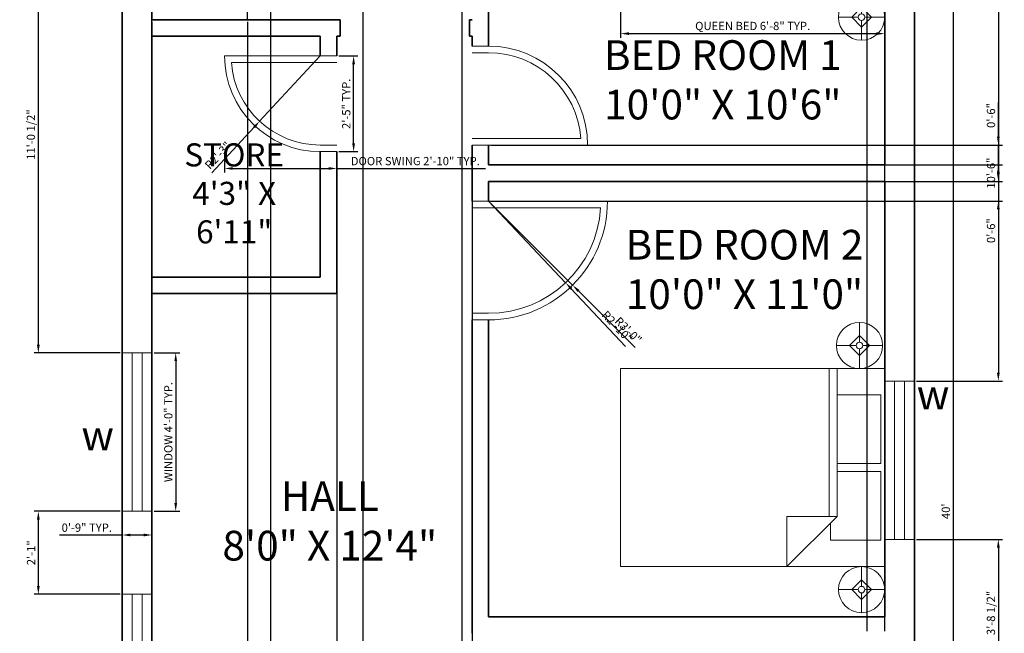
# Model space of a CAD drawing. Units: inches. Extents: x 3796 to 4094, y 4410 to 4948.
# Tile 2 of 3: x 3796 to 4094, y 4640 to 4826. Entities that reach past the tile are written whole.
import ezdxf

# ---------------------------------------------------------------- set-up
doc = ezdxf.new("R2010")
doc.units = ezdxf.units.IN
for name, color, linetype, lineweight in [('A-ANNO-DIMS', 2, 'Continuous', 18), ('A-ANNO-TEXT', 7, 'Continuous', 18), ('A-AREA-IDEN', 7, 'Continuous', 25), ('A-DOOR', 3, 'Continuous', 18), ('A-FLOR-CASE', 8, 'Continuous', 25), ('A-FURN', 8, 'Continuous', 18), ('A-GLAZ', 4, 'Continuous', 18), ('A-WALL', 7, 'Continuous', 35)]:
    doc.layers.add(name, color=color, linetype=linetype, lineweight=lineweight)
doc.styles.get("Standard").update_dxf_attribs({"font": 'arial.ttf'})
doc.dimstyles.new('ISO-25', dxfattribs={"dimtxt": 2.5, "dimasz": 2.5, "dimexe": 1.25, "dimexo": 0.625, "dimtad": 1, "dimdec": 0, "dimlunit": 3, "dimtxsty": 'Standard', "dimcen": 2.5, "dimadec": 0, "dimazin": 0, "dimtfac": 1, "dimtdec": 0, "dimtmove": 0, "dimatfit": 3, "dimfxl": 1, "dimarcsym": 0})

# ---------------------------------------------------------------- blocks, each defined once
blk = doc.blocks.new('*D2')
at = {"layer": 'A-ANNO-DIMS', "color": 0, "lineweight": -2, "transparency": 16777216}
for p, q in [((4067.39, 4916.55), (4079.78, 4916.55)), ((4078.53, 4914.05), (4078.53, 4439.05)), ((4067.39, 4436.55), (4079.78, 4436.55))]:
    blk.add_line(p, q, dxfattribs=at)
at = {"layer": 'A-ANNO-DIMS', "color": 0, "transparency": 16777216}
for points in [[(4078.11, 4914.05), (4078.94, 4914.05), (4078.53, 4916.55)], [(4078.11, 4439.05), (4078.94, 4439.05), (4078.53, 4436.55)]]:
    blk.add_solid(points, dxfattribs=at)
at = {"layer": 'Defpoints', "color": 0, "transparency": 16777216}
for p in [(4066.76, 4916.55), (4066.76, 4436.55), (4078.53, 4436.55)]:
    blk.add_point(p, dxfattribs=at)
at = {"layer": 'A-ANNO-DIMS', "color": 0, "transparency": 16777216, "insert": (4076.62, 4676.55), "char_height": 2.5, "attachment_point": 5, "rotation": 90}
blk.add_mtext("40'", dxfattribs=at)
blk = doc.blocks.new('Lamp - Table')
for p, q in [((0, 7), (0, 1)), ((0, 3), (-3, 0)), ((3, 0), (0, 3)), ((-1, 0), (-7, 0)), ((-3, 0), (0, -3)), ((0, -3), (3, 0)), ((1, 0), (7, 0)), ((0, -1), (0, -7))]:
    blk.add_line(p, q)
for radius in [7, 1]:
    blk.add_circle((0, 0), radius)
blk = doc.blocks.new('Bed - Queen')
for p, q in [((0, -80.00003), (0, 0)), ((0, 0), (59.99999, 0)), ((59.99999, 0), (59.99999, -80.00003)), ((7.99999, -1.2), (28.79998, -1.2)), ((7.99999, -14.4), (7.99999, -1.2)), ((28.79998, -1.2), (28.79998, -14.4)), ((31.19999, -1.2), (51.99999, -1.2)), ((31.19999, -14.4), (31.19999, -1.2)), ((51.99999, -1.2), (51.99999, -16.4)), ((0, -14.4), (44.8, -14.4)), ((59.99999, -29.6), (44.8, -14.4)), ((44.8, -14.4), (44.8, -29.6)), ((44.8, -16.8), (0, -16.8)), ((51.99999, -16.4), (46.79936, -16.4)), ((44.8, -29.6), (59.99999, -29.6)), ((59.99999, -80.00003), (0, -80.00003))]:
    blk.add_line(p, q)
blk = doc.blocks.new('WIN-48IN')
for p, q in [((0, 48), (0, 0)), ((9, 48), (0, 48)), ((3, 48), (3, 0)), ((6, 0), (6, 48)), ((9, 0), (9, 48)), ((0, 0), (9, 0))]:
    blk.add_line(p, q)
blk = doc.blocks.new('DOOR-SWING-29IN')
for p, q in [((0, 0), (-29, 0)), ((0, 0), (5, 0)), ((0, -2), (-26.93, -2)), ((0, -2), (5, -2)), ((5, -27), (0, -27)), ((5, -29), (0, -29))]:
    blk.add_line(p, q)
for radius, start in [(29, 180), (27, 184.248)]:
    blk.add_arc((0, 0), radius, start, 270)
blk = doc.blocks.new('*D11')
at = {"layer": 'A-ANNO-DIMS', "color": 0, "lineweight": -2, "transparency": 16777216}
for p, q in [((3836.39, 4724.55), (3844.21, 4724.55)), ((3842.96, 4722.05), (3842.96, 4679.05)), ((3836.39, 4676.55), (3844.21, 4676.55))]:
    blk.add_line(p, q, dxfattribs=at)
at = {"layer": 'A-ANNO-DIMS', "color": 0, "transparency": 16777216}
for points in [[(3842.55, 4722.05), (3843.38, 4722.05), (3842.96, 4724.55)], [(3842.55, 4679.05), (3843.38, 4679.05), (3842.96, 4676.55)]]:
    blk.add_solid(points, dxfattribs=at)
at = {"layer": 'Defpoints', "color": 0, "transparency": 16777216}
for p in [(3835.76, 4724.55), (3835.76, 4676.55), (3842.96, 4676.55)]:
    blk.add_point(p, dxfattribs=at)
at = {"layer": 'A-ANNO-DIMS', "color": 0, "transparency": 16777216, "insert": (3841.05, 4700.55), "char_height": 2.5, "attachment_point": 5, "rotation": 90}
blk.add_mtext('WINDOW 4\'-0" TYP.', dxfattribs=at)
blk = doc.blocks.new('*D12')
at = {"layer": 'A-ANNO-DIMS', "color": 0, "lineweight": -2, "transparency": 16777216}
for p, q in [((3826.76, 4675.93), (3826.76, 4668.1)), ((3835.76, 4675.93), (3835.76, 4668.1)), ((3826.76, 4669.35), (3807.78, 4669.35)), ((3833.26, 4669.35), (3829.26, 4669.35))]:
    blk.add_line(p, q, dxfattribs=at)
at = {"layer": 'A-ANNO-DIMS', "color": 0, "transparency": 16777216}
for points in [[(3829.26, 4669.77), (3829.26, 4668.94), (3826.76, 4669.35)], [(3833.26, 4669.77), (3833.26, 4668.94), (3835.76, 4669.35)]]:
    blk.add_solid(points, dxfattribs=at)
at = {"layer": 'Defpoints', "color": 0, "transparency": 16777216}
for p in [(3826.76, 4676.55), (3835.76, 4676.55), (3826.76, 4669.35)]:
    blk.add_point(p, dxfattribs=at)
at = {"layer": 'A-ANNO-DIMS', "color": 0, "transparency": 16777216, "insert": (3816.02, 4671.25), "char_height": 2.5, "attachment_point": 5}
blk.add_mtext('0\'-9" TYP.', dxfattribs=at)
blk = doc.blocks.new('*D15')
at = {"layer": 'A-ANNO-DIMS', "color": 0, "lineweight": -2, "transparency": 16777216}
for p, q in [((3977.76, 4832.71), (3977.76, 4820.08)), ((4057.76, 4832.71), (4057.76, 4820.08)), ((3980.26, 4821.33), (4055.26, 4821.33))]:
    blk.add_line(p, q, dxfattribs=at)
at = {"layer": 'A-ANNO-DIMS', "color": 0, "transparency": 16777216}
for points in [[(3980.26, 4821.75), (3980.26, 4820.92), (3977.76, 4821.33)], [(4055.26, 4821.75), (4055.26, 4820.92), (4057.76, 4821.33)]]:
    blk.add_solid(points, dxfattribs=at)
at = {"layer": 'Defpoints', "color": 0, "transparency": 16777216}
for p in [(3977.76, 4833.33), (4057.76, 4833.33), (4057.76, 4821.33)]:
    blk.add_point(p, dxfattribs=at)
at = {"layer": 'A-ANNO-DIMS', "color": 0, "transparency": 16777216, "insert": (4017.76, 4823.33), "char_height": 2.5, "attachment_point": 5}
blk.add_mtext('QUEEN BED 6\'-8" TYP.', dxfattribs=at)
blk = doc.blocks.new('*D19')
at = {"layer": 'A-ANNO-DIMS', "color": 0, "lineweight": -2, "transparency": 16777216}
for p, q in [((3857.76, 4784.93), (3857.76, 4779.2)), ((3891.76, 4784.93), (3891.76, 4779.2)), ((3860.26, 4780.45), (3889.26, 4780.45)), ((3891.76, 4780.45), (3936.82, 4780.45))]:
    blk.add_line(p, q, dxfattribs=at)
at = {"layer": 'A-ANNO-DIMS', "color": 0, "transparency": 16777216}
for points in [[(3860.26, 4780.87), (3860.26, 4780.04), (3857.76, 4780.45)], [(3889.26, 4780.87), (3889.26, 4780.04), (3891.76, 4780.45)]]:
    blk.add_solid(points, dxfattribs=at)
at = {"layer": 'Defpoints', "color": 0, "transparency": 16777216}
for p in [(3857.76, 4785.55), (3891.76, 4785.55), (3891.76, 4780.45)]:
    blk.add_point(p, dxfattribs=at)
at = {"layer": 'A-ANNO-DIMS', "color": 0, "transparency": 16777216, "insert": (3915.54, 4782.37), "char_height": 2.5, "attachment_point": 5}
blk.add_mtext('DOOR SWING 2\'-10" TYP.', dxfattribs=at)
blk = doc.blocks.new('*D20')
at = {"layer": 'A-ANNO-DIMS', "color": 0, "lineweight": -2, "transparency": 16777216}
for p, q in [((3892.39, 4814.55), (3898.11, 4814.55)), ((3896.86, 4788.05), (3896.86, 4812.05)), ((3892.39, 4785.55), (3898.11, 4785.55))]:
    blk.add_line(p, q, dxfattribs=at)
at = {"layer": 'A-ANNO-DIMS', "color": 0, "transparency": 16777216}
for points in [[(3896.45, 4812.05), (3897.28, 4812.05), (3896.86, 4814.55)], [(3896.45, 4788.05), (3897.28, 4788.05), (3896.86, 4785.55)]]:
    blk.add_solid(points, dxfattribs=at)
at = {"layer": 'Defpoints', "color": 0, "transparency": 16777216}
for p in [(3891.76, 4814.55), (3896.86, 4814.55), (3891.76, 4785.55)]:
    blk.add_point(p, dxfattribs=at)
at = {"layer": 'A-ANNO-DIMS', "color": 0, "transparency": 16777216, "insert": (3894.96, 4800.05), "char_height": 2.5, "attachment_point": 5, "rotation": 90}
blk.add_mtext('2\'-5" TYP.', dxfattribs=at)
blk = doc.blocks.new('*D31')
at = {"layer": 'A-ANNO-DIMS', "color": 0, "lineweight": -2, "transparency": 16777216}
for p, q in [((3835.76, 4482.18), (3835.76, 4943.23)), ((3871.76, 4490.18), (3871.76, 4943.23)), ((3838.26, 4941.98), (3869.26, 4941.98))]:
    blk.add_line(p, q, dxfattribs=at)
at = {"layer": 'A-ANNO-DIMS', "color": 0, "transparency": 16777216}
for points in [[(3838.26, 4942.39), (3838.26, 4941.56), (3835.76, 4941.98)], [(3869.26, 4942.39), (3869.26, 4941.56), (3871.76, 4941.98)]]:
    blk.add_solid(points, dxfattribs=at)
at = {"layer": 'Defpoints', "color": 0, "transparency": 16777216}
for p in [(3871.76, 4941.98), (3871.76, 4489.55), (3835.76, 4481.55)]:
    blk.add_point(p, dxfattribs=at)
at = {"layer": 'A-ANNO-DIMS', "color": 0, "transparency": 16777216, "insert": (3853.76, 4943.88), "char_height": 2.5, "attachment_point": 5}
blk.add_mtext('3\'-0"', dxfattribs=at)
blk = doc.blocks.new('*D34')
at = {"layer": 'A-ANNO-DIMS', "color": 0, "lineweight": -2, "transparency": 16777216}
for p, q in [((3899.76, 4580.18), (3899.76, 4943.23)), ((3929.76, 4580.18), (3929.76, 4943.23)), ((3902.26, 4941.98), (3927.26, 4941.98))]:
    blk.add_line(p, q, dxfattribs=at)
at = {"layer": 'A-ANNO-DIMS', "color": 0, "transparency": 16777216}
for points in [[(3902.26, 4942.39), (3902.26, 4941.56), (3899.76, 4941.98)], [(3927.26, 4942.39), (3927.26, 4941.56), (3929.76, 4941.98)]]:
    blk.add_solid(points, dxfattribs=at)
at = {"layer": 'Defpoints', "color": 0, "transparency": 16777216}
for p in [(3929.76, 4941.98), (3899.76, 4579.55), (3929.76, 4579.55)]:
    blk.add_point(p, dxfattribs=at)
at = {"layer": 'A-ANNO-DIMS', "color": 0, "transparency": 16777216, "insert": (3914.76, 4943.88), "char_height": 2.5, "attachment_point": 5}
blk.add_mtext('2\'-6"', dxfattribs=at)
blk = doc.blocks.new('*D38')
at = {"layer": 'A-ANNO-DIMS', "color": 0, "lineweight": -2, "transparency": 16777216}
for p, q in [((3826.14, 4856.88), (3800.09, 4856.88)), ((3801.34, 4854.38), (3801.34, 4727.05)), ((3826.14, 4724.55), (3800.09, 4724.55))]:
    blk.add_line(p, q, dxfattribs=at)
at = {"layer": 'A-ANNO-DIMS', "color": 0, "transparency": 16777216}
for points in [[(3800.92, 4854.38), (3801.76, 4854.38), (3801.34, 4856.88)], [(3800.92, 4727.05), (3801.76, 4727.05), (3801.34, 4724.55)]]:
    blk.add_solid(points, dxfattribs=at)
at = {"layer": 'Defpoints', "color": 0, "transparency": 16777216}
for p in [(3826.76, 4856.88), (3801.34, 4724.55), (3826.76, 4724.55)]:
    blk.add_point(p, dxfattribs=at)
at = {"layer": 'A-ANNO-DIMS', "color": 0, "transparency": 16777216, "insert": (3799.42, 4790.72), "char_height": 2.5, "attachment_point": 5, "rotation": 90}
blk.add_mtext('11\'-0 1/2"', dxfattribs=at)
blk = doc.blocks.new('*D39')
at = {"layer": 'A-ANNO-DIMS', "color": 0, "lineweight": -2, "transparency": 16777216}
for p, q in [((3826.14, 4676.55), (3800.09, 4676.55)), ((3801.34, 4674.05), (3801.34, 4653.89)), ((3826.14, 4651.39), (3800.09, 4651.39))]:
    blk.add_line(p, q, dxfattribs=at)
at = {"layer": 'A-ANNO-DIMS', "color": 0, "transparency": 16777216}
for points in [[(3800.92, 4674.05), (3801.76, 4674.05), (3801.34, 4676.55)], [(3800.92, 4653.89), (3801.76, 4653.89), (3801.34, 4651.39)]]:
    blk.add_solid(points, dxfattribs=at)
at = {"layer": 'Defpoints', "color": 0, "transparency": 16777216}
for p in [(3826.76, 4676.55), (3801.34, 4651.39), (3826.76, 4651.39)]:
    blk.add_point(p, dxfattribs=at)
at = {"layer": 'A-ANNO-DIMS', "color": 0, "transparency": 16777216, "insert": (3799.46, 4663.97), "char_height": 2.5, "attachment_point": 5, "rotation": 90}
blk.add_mtext('2\'-1"', dxfattribs=at)
blk = doc.blocks.new('*D41')
at = {"layer": 'A-ANNO-DIMS', "color": 0, "lineweight": -2, "transparency": 16777216}
for p, q in [((4067.39, 4842.05), (4093.44, 4842.05)), ((4092.19, 4839.55), (4092.19, 4718.53)), ((4067.39, 4716.03), (4093.44, 4716.03))]:
    blk.add_line(p, q, dxfattribs=at)
at = {"layer": 'A-ANNO-DIMS', "color": 0, "transparency": 16777216}
for points in [[(4091.77, 4839.55), (4092.61, 4839.55), (4092.19, 4842.05)], [(4091.77, 4718.53), (4092.61, 4718.53), (4092.19, 4716.03)]]:
    blk.add_solid(points, dxfattribs=at)
at = {"layer": 'Defpoints', "color": 0, "transparency": 16777216}
for p in [(4066.76, 4842.05), (4066.76, 4716.03), (4092.19, 4716.03)]:
    blk.add_point(p, dxfattribs=at)
at = {"layer": 'A-ANNO-DIMS', "color": 0, "transparency": 16777216, "insert": (4090.29, 4779.04), "char_height": 2.5, "attachment_point": 5, "rotation": 90}
blk.add_mtext('10\'-6"', dxfattribs=at)
blk = doc.blocks.new('*D42')
at = {"layer": 'A-ANNO-DIMS', "color": 0, "lineweight": -2, "transparency": 16777216}
for p, q in [((4067.39, 4668.03), (4093.44, 4668.03)), ((4092.19, 4665.53), (4092.19, 4625.92)), ((4067.39, 4623.42), (4093.44, 4623.42))]:
    blk.add_line(p, q, dxfattribs=at)
at = {"layer": 'A-ANNO-DIMS', "color": 0, "transparency": 16777216}
for points in [[(4091.77, 4665.53), (4092.61, 4665.53), (4092.19, 4668.03)], [(4091.77, 4625.92), (4092.61, 4625.92), (4092.19, 4623.42)]]:
    blk.add_solid(points, dxfattribs=at)
at = {"layer": 'Defpoints', "color": 0, "transparency": 16777216}
for p in [(4066.76, 4668.03), (4066.76, 4623.42), (4092.19, 4623.42)]:
    blk.add_point(p, dxfattribs=at)
at = {"layer": 'A-ANNO-DIMS', "color": 0, "transparency": 16777216, "insert": (4090.27, 4645.73), "char_height": 2.5, "attachment_point": 5, "rotation": 90}
blk.add_mtext('3\'-8 1/2"', dxfattribs=at)
blk = doc.blocks.new('*D45')
at = {"layer": 'A-ANNO-DIMS', "color": 0, "lineweight": -2, "transparency": 16777216}
for p, q in [((3835.76, 4824.93), (3835.76, 4409.83)), ((3864.76, 4824.93), (3864.76, 4409.83)), ((3862.26, 4411.08), (3838.26, 4411.08))]:
    blk.add_line(p, q, dxfattribs=at)
at = {"layer": 'A-ANNO-DIMS', "color": 0, "transparency": 16777216}
for points in [[(3838.26, 4411.49), (3838.26, 4410.66), (3835.76, 4411.08)], [(3862.26, 4411.49), (3862.26, 4410.66), (3864.76, 4411.08)]]:
    blk.add_solid(points, dxfattribs=at)
at = {"layer": 'Defpoints', "color": 0, "transparency": 16777216}
for p in [(3835.76, 4825.55), (3864.76, 4825.55), (3835.76, 4411.08)]:
    blk.add_point(p, dxfattribs=at)
at = {"layer": 'A-ANNO-DIMS', "color": 0, "transparency": 16777216, "insert": (3850.26, 4412.98), "char_height": 2.5, "attachment_point": 5}
blk.add_mtext('2\'-5"', dxfattribs=at)
blk = doc.blocks.new('*D48')
at = {"layer": 'A-ANNO-DIMS', "color": 0, "lineweight": -2, "transparency": 16777216}
for p, q in [((4052.41, 4640.18), (4052.41, 4943.23)), ((4057.76, 4640.18), (4057.76, 4943.23)), ((4049.91, 4941.98), (4047.41, 4941.98)), ((4052.41, 4941.98), (4057.76, 4941.98)), ((4060.26, 4941.98), (4076.49, 4941.98))]:
    blk.add_line(p, q, dxfattribs=at)
at = {"layer": 'A-ANNO-DIMS', "color": 0, "transparency": 16777216}
for points in [[(4049.91, 4942.39), (4049.91, 4941.56), (4052.41, 4941.98)], [(4060.26, 4942.39), (4060.26, 4941.56), (4057.76, 4941.98)]]:
    blk.add_solid(points, dxfattribs=at)
at = {"layer": 'Defpoints', "color": 0, "transparency": 16777216}
for p in [(4057.76, 4941.98), (4052.41, 4639.55), (4057.76, 4639.55)]:
    blk.add_point(p, dxfattribs=at)
at = {"layer": 'A-ANNO-DIMS', "color": 0, "transparency": 16777216, "insert": (4069.62, 4943.9), "char_height": 2.5, "attachment_point": 5}
blk.add_mtext('0\'-5 1/2"', dxfattribs=at)
blk = doc.blocks.new('*D51')
at = {"layer": 'A-ANNO-DIMS', "color": 0, "lineweight": -2, "transparency": 16777216}
for p, q in [((4092.19, 4790.05), (4092.19, 4800.45)), ((3938.39, 4787.55), (4093.44, 4787.55)), ((4092.19, 4781.55), (4092.19, 4787.55)), ((3938.39, 4781.55), (4093.44, 4781.55)), ((4092.19, 4779.05), (4092.19, 4776.55))]:
    blk.add_line(p, q, dxfattribs=at)
at = {"layer": 'A-ANNO-DIMS', "color": 0, "transparency": 16777216}
for points in [[(4091.77, 4790.05), (4092.61, 4790.05), (4092.19, 4787.55)], [(4091.77, 4779.05), (4092.61, 4779.05), (4092.19, 4781.55)]]:
    blk.add_solid(points, dxfattribs=at)
at = {"layer": 'Defpoints', "color": 0, "transparency": 16777216}
for p in [(3937.76, 4787.55), (4092.19, 4787.55), (3937.76, 4781.55)]:
    blk.add_point(p, dxfattribs=at)
at = {"layer": 'A-ANNO-DIMS', "color": 0, "transparency": 16777216, "insert": (4090.29, 4796.5), "char_height": 2.5, "attachment_point": 5, "rotation": 90}
blk.add_mtext('0\'-6"', dxfattribs=at)
blk = doc.blocks.new('*D52')
at = {"layer": 'A-ANNO-DIMS', "color": 0, "lineweight": -2, "transparency": 16777216}
for p, q in [((4092.19, 4779.05), (4092.19, 4781.55)), ((3938.39, 4776.55), (4093.44, 4776.55)), ((4092.19, 4776.55), (4092.19, 4770.55)), ((3938.39, 4770.55), (4093.44, 4770.55)), ((4092.19, 4768.05), (4092.19, 4757.66))]:
    blk.add_line(p, q, dxfattribs=at)
at = {"layer": 'A-ANNO-DIMS', "color": 0, "transparency": 16777216}
for points in [[(4091.77, 4779.05), (4092.61, 4779.05), (4092.19, 4776.55)], [(4091.77, 4768.05), (4092.61, 4768.05), (4092.19, 4770.55)]]:
    blk.add_solid(points, dxfattribs=at)
at = {"layer": 'Defpoints', "color": 0, "transparency": 16777216}
for p in [(3937.76, 4776.55), (3937.76, 4770.55), (4092.19, 4770.55)]:
    blk.add_point(p, dxfattribs=at)
at = {"layer": 'A-ANNO-DIMS', "color": 0, "transparency": 16777216, "insert": (4090.29, 4761.6), "char_height": 2.5, "attachment_point": 5, "rotation": 90}
blk.add_mtext('0\'-6"', dxfattribs=at)
blk = doc.blocks.new('*D54')
at = {"layer": 'A-ANNO-DIMS', "color": 0, "lineweight": -2, "transparency": 16777216}
for p, q in [((3891.76, 4784.93), (3891.76, 4409.83)), ((3932.76, 4786.93), (3932.76, 4409.83)), ((3894.26, 4411.08), (3930.26, 4411.08))]:
    blk.add_line(p, q, dxfattribs=at)
at = {"layer": 'A-ANNO-DIMS', "color": 0, "transparency": 16777216}
for points in [[(3894.26, 4411.49), (3894.26, 4410.66), (3891.76, 4411.08)], [(3930.26, 4411.49), (3930.26, 4410.66), (3932.76, 4411.08)]]:
    blk.add_solid(points, dxfattribs=at)
at = {"layer": 'Defpoints', "color": 0, "transparency": 16777216}
for p in [(3891.76, 4785.55), (3932.76, 4787.55), (3932.76, 4411.08)]:
    blk.add_point(p, dxfattribs=at)
at = {"layer": 'A-ANNO-DIMS', "color": 0, "transparency": 16777216, "insert": (3912.26, 4412.98), "char_height": 2.5, "attachment_point": 5}
blk.add_mtext('3\'-5"', dxfattribs=at)
blk = doc.blocks.new('*D55')
at = {"layer": 'A-ANNO-DIMS', "color": 0, "lineweight": -2, "transparency": 16777216}
for p, q in [((3937.76, 4770.55), (3963.22, 4745.1)), ((3982.13, 4726.19), (3964.99, 4743.33))]:
    blk.add_line(p, q, dxfattribs=at)
at = {"layer": 'A-ANNO-DIMS', "color": 0, "transparency": 16777216}
blk.add_solid([(3965.28, 4743.62), (3964.69, 4743.03), (3963.22, 4745.1)], dxfattribs=at)
at = {"layer": 'Defpoints', "color": 0, "transparency": 16777216}
for p in [(3937.76, 4770.55), (3963.22, 4745.1)]:
    blk.add_point(p, dxfattribs=at)
at = {"layer": 'A-ANNO-DIMS', "color": 0, "transparency": 16777216, "insert": (3979.84, 4731.17), "char_height": 2.5, "attachment_point": 5, "rotation": 315.0005}
blk.add_mtext('R3\'-0"', dxfattribs=at)
blk = doc.blocks.new('*D56')
at = {"layer": 'A-ANNO-DIMS', "color": 0, "lineweight": -2, "transparency": 16777216}
for p, q in [((3937.76, 4770.55), (3961.09, 4745.81)), ((3979.28, 4726.52), (3962.8, 4743.99))]:
    blk.add_line(p, q, dxfattribs=at)
at = {"layer": 'A-ANNO-DIMS', "color": 0, "transparency": 16777216}
blk.add_solid([(3963.11, 4744.28), (3962.5, 4743.71), (3961.09, 4745.81)], dxfattribs=at)
at = {"layer": 'Defpoints', "color": 0, "transparency": 16777216}
for p in [(3937.76, 4770.55), (3961.09, 4745.81)]:
    blk.add_point(p, dxfattribs=at)
at = {"layer": 'A-ANNO-DIMS', "color": 0, "transparency": 16777216, "insert": (3976.47, 4732.28), "char_height": 2.5, "attachment_point": 5, "rotation": 313.3141}
blk.add_mtext('R2\'-10"', dxfattribs=at)
blk = doc.blocks.new('*D61')
at = {"layer": 'A-ANNO-DIMS', "color": 0, "lineweight": -2, "transparency": 16777216}
for p, q in [((3886.76, 4814.55), (3868.39, 4794.77)), ((3853.87, 4779.12), (3866.69, 4792.93))]:
    blk.add_line(p, q, dxfattribs=at)
at = {"layer": 'A-ANNO-DIMS', "color": 0, "transparency": 16777216}
blk.add_solid([(3866.39, 4793.22), (3867, 4792.65), (3868.39, 4794.77)], dxfattribs=at)
at = {"layer": 'Defpoints', "color": 0, "transparency": 16777216}
for p in [(3886.76, 4814.55), (3868.39, 4794.77)]:
    blk.add_point(p, dxfattribs=at)
at = {"layer": 'A-ANNO-DIMS', "color": 0, "transparency": 16777216, "insert": (3855.98, 4784.19), "char_height": 2.5, "attachment_point": 5, "rotation": 47.1241}
blk.add_mtext('R2\'-3"', dxfattribs=at)

msp = doc.modelspace()

# ---------------------------------------------------------------- linework, layer by layer
at = {"layer": 'A-DOOR'}
for p, q in [((3932.76, 4817.55), (3937.76, 4817.55)), ((3932.76, 4815.55), (3937.76, 4815.55)), ((3937.76, 4789.55), (3932.76, 4789.55)), ((3937.76, 4789.55), (3965.69, 4789.55)), ((3937.76, 4787.55), (3932.76, 4787.55)), ((3937.76, 4787.55), (3967.76, 4787.55)), ((3937.76, 4770.55), (3932.76, 4770.55)), ((3937.76, 4770.55), (3973.76, 4770.55)), ((3937.76, 4768.55), (3932.76, 4768.55)), ((3937.76, 4768.55), (3971.71, 4768.55)), ((3932.76, 4736.55), (3937.76, 4736.55)), ((3932.76, 4734.55), (3937.76, 4734.55))]:
    msp.add_line(p, q, dxfattribs=at)
for centre, radius, start, end in [((3937.76, 4787.55), 30, 0, 90), ((3937.76, 4787.55), 28, 4.096, 90), ((3937.76, 4770.55), 36, 270, 0), ((3937.76, 4770.55), 34, 270, 356.6277)]:
    msp.add_arc(centre, radius, start, end, dxfattribs=at)
at = {"layer": 'A-FLOR-CASE'}
msp.add_line((3864.76, 4825.55), (3864.76, 4878.55), dxfattribs=at)
at = {"layer": 'A-WALL'}
for p, q in [((3826.76, 4436.55), (3826.76, 4916.55)), ((4066.76, 4916.55), (4066.76, 4436.55)), ((3835.76, 4825.55), (3835.76, 4907.55)), ((3937.76, 4907.55), (3937.76, 4817.55)), ((3937.76, 4817.55), (3937.76, 4907.55)), ((4057.76, 4907.55), (4057.76, 4781.55)), ((3835.76, 4825.55), (3892.75, 4825.55)), ((3892.75, 4820.55), (3892.75, 4825.55)), ((3932.02, 4825.55), (3932.02, 4820.55)), ((3932.02, 4825.55), (3932.76, 4825.55)), ((3835.76, 4820.55), (3886.76, 4820.55)), ((3835.76, 4747.55), (3835.76, 4820.55)), ((3886.76, 4820.55), (3886.76, 4814.55)), ((3886.76, 4814.55), (3886.76, 4820.55)), ((3891.76, 4820.55), (3892.75, 4820.55)), ((3891.76, 4820.55), (3892.75, 4820.55)), ((3891.76, 4814.55), (3891.76, 4820.55)), ((3932.02, 4820.55), (3932.76, 4820.55)), ((3932.76, 4820.55), (3932.76, 4817.55)), ((3886.76, 4747.55), (3886.76, 4785.55)), ((3891.76, 4742.55), (3891.76, 4785.55)), ((3932.76, 4787.55), (3932.76, 4770.55)), ((3937.76, 4781.55), (3937.76, 4787.55)), ((3937.76, 4781.55), (3937.76, 4787.55)), ((3937.76, 4787.55), (3937.76, 4781.55)), ((3937.76, 4781.55), (4057.76, 4781.55)), ((3937.76, 4776.55), (4057.76, 4776.55)), ((3937.76, 4776.55), (3937.76, 4770.55)), ((3937.76, 4776.55), (3937.76, 4770.55)), ((3937.76, 4770.55), (3937.76, 4776.55)), ((4057.76, 4776.55), (4057.76, 4644.55)), ((3835.76, 4747.55), (3886.76, 4747.55)), ((3835.76, 4742.55), (3891.76, 4742.55)), ((3835.76, 4584.55), (3835.76, 4742.55)), ((3932.76, 4734.55), (3932.76, 4639.55)), ((3937.76, 4644.55), (3937.76, 4734.55)), ((3937.76, 4734.55), (3937.76, 4644.55)), ((3937.76, 4644.55), (4057.76, 4644.55))]:
    msp.add_line(p, q, dxfattribs=at)

# ---------------------------------------------------------------- block references
at = {"layer": 'A-DOOR'}
msp.add_blockref('DOOR-SWING-29IN', (3886.76, 4814.55), dxfattribs=at)
at = {"layer": 'A-FURN', "rotation": 270}
for name, p in [('Lamp - Table', (4050.76, 4826.33)), ('Lamp - Table', (4050.13, 4726.79)), ('Bed - Queen', (4057.76, 4719.79)), ('Lamp - Table', (4050.77, 4652.79))]:
    msp.add_blockref(name, p, dxfattribs=at)
at = {"layer": 'A-GLAZ', "rotation": 180}
for p in [(3835.76, 4724.55), (4066.76, 4716.03), (3835.76, 4651.39)]:
    msp.add_blockref('WIN-48IN', p, dxfattribs=at)

# ---------------------------------------------------------------- texts
at = {"layer": 'A-ANNO-TEXT', "char_height": 9, "attachment_point": 1}
for insert in [(4042.95, 4716.4), (3789.85, 4704.04)]:
    msp.add_mtext_dynamic_manual_height_columns('\\pxqc;w', width=58.9432, gutter_width=12.5, heights=[0], dxfattribs=dict(at, insert=insert))
at = {"layer": 'A-AREA-IDEN', "attachment_point": 1}
for s, width, insert, char_height in [('\\pxqc;BED ROOM 1\\P10\'0" X 10\'6"', 98.0813, (3959.68, 4819.32), 9), ('\\pxqc;STORE\\P4\'3" X 6\'11"', 49.8486, (3835.76, 4788.07), 7), ('\\pxqc;BED ROOM 2\\P10\'0" X 11\'0"', 93.027, (3968.77, 4761.84), 9), ('\\pxqc;HALL\\P8\'0" X 12\'4"', 74.3063, (3852.5, 4685.62), 9)]:
    msp.add_mtext_dynamic_manual_height_columns(s, width=width, gutter_width=12.5, heights=[0], dxfattribs=dict(at, insert=insert, char_height=char_height))

# ---------------------------------------------------------------- dimensions: what is measured, and where the dimension line sits
at = {"layer": 'A-ANNO-DIMS'}
for base, p1, p2, picture, middle in [((4057.7642, 4941.9774), (4052.4081, 4639.5524), (4057.7642, 4639.5524), '*D48', (4069.6247, 4943.8951)), ((3871.76, 4941.98), (3835.76, 4481.55), (3871.76, 4489.55), '*D31', (3853.76, 4943.88)), ((3929.76, 4941.98), (3899.76, 4579.55), (3929.76, 4579.55), '*D34', (3914.76, 4943.88)), ((3835.76, 4411.08), (3864.76, 4825.55), (3835.76, 4825.55), '*D45', (3850.26, 4412.98)), ((3932.76, 4411.08), (3891.76, 4785.55), (3932.76, 4787.55), '*D54', (3912.26, 4412.98))]:
    dim = msp.add_linear_dim(base=base, p1=p1, p2=p2, dimstyle='ISO-25', override={"dimdec": 1, "dimlfac": 1, "dimrnd": 0, "dimzin": 1, "dimdsep": 46, "dimlunit": 4, "dimfrac": 2}, dxfattribs=at)
    dim.commit()
    dim.dimension.update_dxf_attribs({"geometry": picture, "text_midpoint": middle})
for base, p1, p2, override, picture, middle in [((4078.53, 4436.55), (4066.76, 4916.55), (4066.76, 4436.55), {"dimclrd": 0, "dimclre": 0, "dimclrt": 0}, '*D2', (4076.62, 4676.55)), ((3801.34, 4724.55), (3826.76, 4856.88), (3826.76, 4724.55), {"dimdec": 1, "dimlfac": 1, "dimrnd": 0, "dimzin": 1, "dimdsep": 46, "dimlunit": 4, "dimfrac": 2}, '*D38', (3799.42, 4790.72)), ((4092.19, 4716.03), (4066.76, 4842.05), (4066.76, 4716.03), {"dimdec": 1, "dimlfac": 1, "dimrnd": 0, "dimzin": 1, "dimdsep": 46, "dimlunit": 4, "dimfrac": 2}, '*D41', (4090.29, 4779.04)), ((4092.19, 4787.55), (3937.76, 4781.55), (3937.76, 4787.55), {"dimdec": 1, "dimlfac": 1, "dimrnd": 0, "dimzin": 1, "dimdsep": 46, "dimlunit": 4, "dimfrac": 2}, '*D51', (4090.29, 4796.5)), ((4092.19, 4770.55), (3937.76, 4776.55), (3937.76, 4770.55), {"dimdec": 1, "dimlfac": 1, "dimrnd": 0, "dimzin": 1, "dimdsep": 46, "dimlunit": 4, "dimfrac": 2}, '*D52', (4090.29, 4761.6)), ((3801.34, 4651.39), (3826.76, 4676.55), (3826.76, 4651.39), {"dimdec": 1, "dimlfac": 1, "dimrnd": 0, "dimzin": 1, "dimdsep": 46, "dimlunit": 4, "dimfrac": 2}, '*D39', (3799.46, 4663.97)), ((4092.19, 4623.42), (4066.76, 4668.03), (4066.76, 4623.42), {"dimdec": 1, "dimlfac": 1, "dimrnd": 0, "dimzin": 1, "dimdsep": 46, "dimlunit": 4, "dimfrac": 2}, '*D42', (4090.27, 4645.73))]:
    dim = msp.add_linear_dim(base=base, p1=p1, p2=p2, angle=90, dimstyle='ISO-25', override=override, dxfattribs=at)
    dim.commit()
    dim.dimension.update_dxf_attribs({"geometry": picture, "text_midpoint": middle})
for base, p1, p2, text, picture, middle in [((4057.76, 4821.33), (3977.76, 4833.33), (4057.76, 4833.33), 'QUEEN BED <> TYP.', '*D15', (4017.76, 4823.33)), ((3891.76, 4780.45), (3857.76, 4785.55), (3891.76, 4785.55), 'DOOR SWING <> TYP.', '*D19', (3915.54, 4782.37))]:
    dim = msp.add_linear_dim(base=base, p1=p1, p2=p2, text=text, dimstyle='ISO-25', override={"dimdec": 1, "dimlfac": 1, "dimrnd": 0, "dimzin": 1, "dimdsep": 46, "dimlunit": 4, "dimfrac": 2}, dxfattribs=at)
    dim.commit()
    dim.dimension.update_dxf_attribs({"geometry": picture, "text_midpoint": middle})
for center, mpoint, picture, middle in [((3886.76, 4814.55), (3868.39, 4794.77), '*D61', (3857.37, 4782.89)), ((3937.76, 4770.55), (3963.22, 4745.1), '*D55', (3978.49, 4729.82)), ((3937.76, 4770.55), (3961.09, 4745.81), '*D56', (3975.08, 4730.97))]:
    dim = msp.add_radius_dim(center=center, mpoint=mpoint, dimstyle='ISO-25', override={"dimdec": 1, "dimlfac": 1, "dimrnd": 0, "dimzin": 1, "dimdsep": 46, "dimlunit": 4, "dimfrac": 2}, dxfattribs=at)
    dim.commit()
    dim.dimension.update_dxf_attribs({"geometry": picture, "text_midpoint": middle, "dimtype": 164})
for base, p1, p2, angle, text, picture, middle in [((3896.86, 4814.55), (3891.76, 4785.55), (3891.76, 4814.55), 90, '<> TYP.', '*D20', (3894.96, 4800.05)), ((3842.96, 4676.55), (3835.76, 4724.55), (3835.76, 4676.55), 270, 'WINDOW <> TYP.', '*D11', (3841.05, 4700.55)), ((3826.76, 4669.35), (3835.76, 4676.55), (3826.76, 4676.55), 180, '<> TYP.', '*D12', (3816.02, 4671.25))]:
    dim = msp.add_linear_dim(base=base, p1=p1, p2=p2, angle=angle, text=text, dimstyle='ISO-25', override={"dimdec": 1, "dimlfac": 1, "dimrnd": 0, "dimzin": 1, "dimdsep": 46, "dimlunit": 4, "dimfrac": 2}, dxfattribs=at)
    dim.commit()
    dim.dimension.update_dxf_attribs({"geometry": picture, "text_midpoint": middle})

doc.saveas('drawing.dxf')
